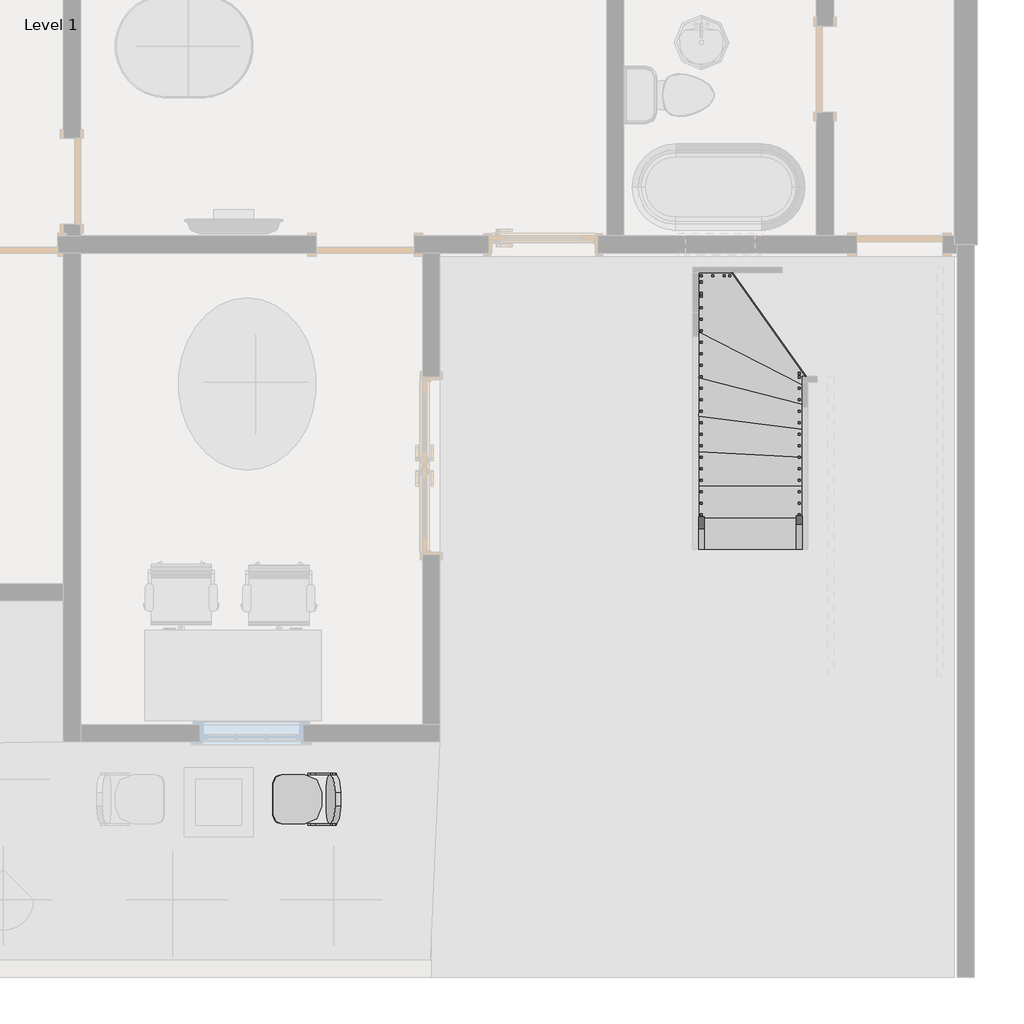
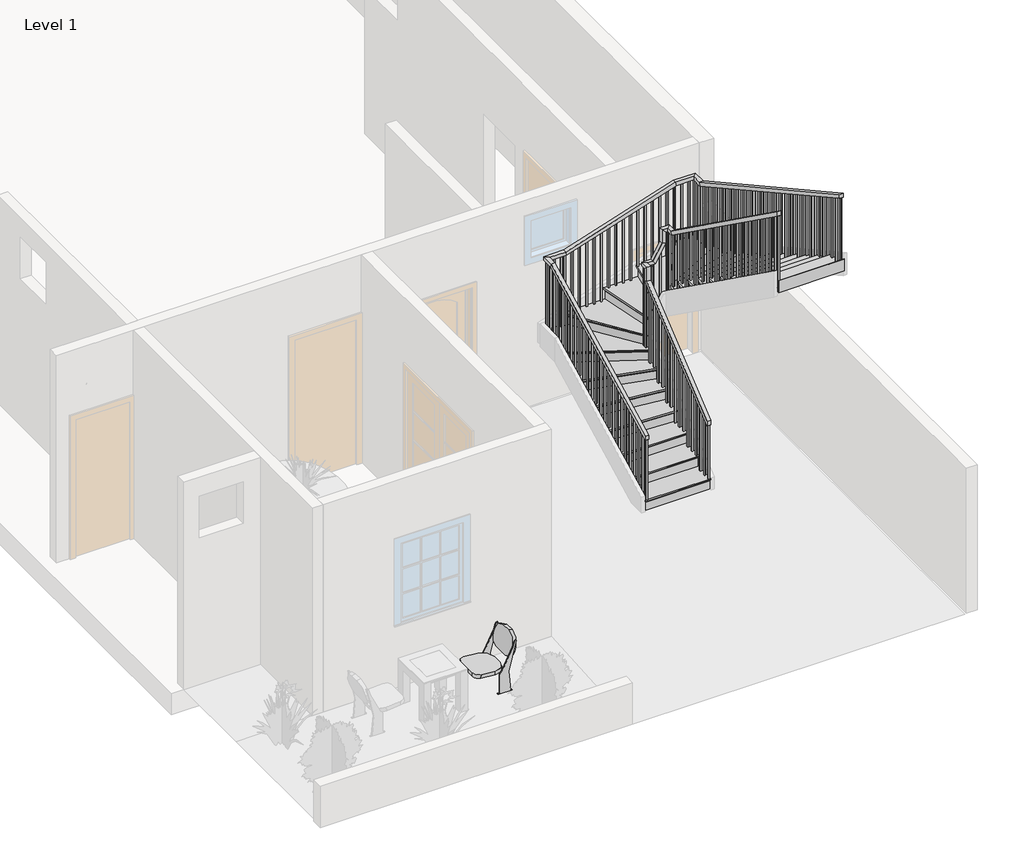
# One storey, part 2 of 3: 2 railings, 1 furniture element, 1 stair flight.
"""IFC4 building model written with IfcOpenShell, lengths in millimetres."""

from ifc_helpers import new_model, si_unit, frame, origin, place, context, project, spatial, polyline, outline, extrude, faceted_brep, transform, mapped, element, save
from components import furniture_3d1d9cbc, stair_flight_43e61283

model = new_model("IFC4")

# Units and contexts
model_context = context("Model", 3, world=origin())
ifc_project = project(units=[si_unit("LENGTHUNIT", "METRE", prefix="MILLI")], contexts=[model_context])

# Site, building, storey
site = spatial("IfcSite", under=ifc_project)
building = spatial("IfcBuilding", under=site)
storey = spatial("IfcBuildingStorey", under=building, Name="Level 1", Elevation=0.0)

# Furniture
placement = place(None, origin())
furniture_shape = furniture_3d1d9cbc(model_context)
element("IfcFurniture", 1, ObjectType="Seating-Auditorium : 18\" x 24\" x 30\"", at=placement, inside=storey, context=model_context, shape_type="MappedRepresentation", body=[
    mapped(furniture_shape, transform((-11062.1267733, -4008.1174688, 0.0), x_axis=(0.0, 1.0, 0.0), y_axis=(-1.0, 0.0, 0.0), z_axis=(0.0, 0.0, 1.0))),
])

# Railings
element("IfcRailing", 2, ObjectType="Handrail - Rectangular", at=placement, inside=storey, context=model_context, shape_type="SolidModel", body=[
    faceted_brep([(-6934.0021832, -1637.5895999, 1025.2529681), (-6934.0021832, -1637.5895999, 959.7067088), (-6883.2021832, -1637.5895999, 959.7067088), (-6883.2021832, -1637.5895999, 1025.2529681), (-6934.0021832, -186.057908, 2208.7848338), (-6934.0021832, -135.257908, 2184.659247), (-6883.2021832, -135.257908, 2184.659247), (-6883.2021832, -186.057908, 2208.7848338), (-6934.0021832, -186.057908, 2414.6281882), (-6934.0021832, -135.257908, 2363.8281882), (-6883.2021832, -135.257908, 2363.8281882), (-6883.2021832, -186.057908, 2414.6281882), (-6934.0021832, -59.057908, 2414.6281882), (-6934.0021832, -59.057908, 2363.8281882), (-6883.2021832, -109.857908, 2363.8281882), (-6883.2021832, -109.857908, 2414.6281882), (-6807.0021832, -59.057908, 2414.6281882), (-6777.8808493, -59.057908, 2363.8281882), (-6777.8808493, -109.857908, 2363.8281882), (-6807.0021832, -109.857908, 2414.6281882), (-6680.0021832, -59.057908, 2631.5051451), (-6629.2021832, -59.057908, 2617.7256424), (-6629.2021832, -109.857908, 2617.7256424), (-6680.0021832, -109.857908, 2631.5051451), (-6680.0021832, -59.057908, 2830.0317636), (-6629.2021832, -59.057908, 2779.2317636), (-6629.2021832, -109.857908, 2779.2317636), (-6680.0021832, -109.857908, 2830.0317636), (-6553.0021832, -59.057908, 2830.0317636), (-6553.0021832, -59.057908, 2779.2317636), (-6603.8021832, -109.857908, 2779.2317636), (-6603.8021832, -109.857908, 2830.0317636), (-6553.0021832, -186.057908, 2830.0317636), (-6553.0021832, -202.3767503, 2779.2317636), (-6603.8021832, -202.3767503, 2779.2317636), (-6603.8021832, -186.057908, 2830.0317636), (-6553.0021832, -2755.1895999, 4670.5627033), (-6603.8021832, -2755.1895999, 4670.5627033), (-6603.8021832, -2755.1895999, 4608.071853), (-6553.0021832, -2755.1895999, 4608.071853)], [[[0, 1, 2, 3]], [[1, 0, 4, 5]], [[2, 1, 5, 6]], [[3, 2, 6, 7]], [[0, 3, 7, 4]], [[5, 4, 8, 9]], [[6, 5, 9, 10]], [[7, 6, 10, 11]], [[4, 7, 11, 8]], [[9, 8, 12, 13]], [[10, 9, 13, 14]], [[11, 10, 14, 15]], [[8, 11, 15, 12]], [[13, 12, 16, 17]], [[14, 13, 17, 18]], [[15, 14, 18, 19]], [[12, 15, 19, 16]], [[17, 16, 20, 21]], [[18, 17, 21, 22]], [[19, 18, 22, 23]], [[16, 19, 23, 20]], [[21, 20, 24, 25]], [[22, 21, 25, 26]], [[23, 22, 26, 27]], [[20, 23, 27, 24]], [[25, 24, 28, 29]], [[26, 25, 29, 30]], [[27, 26, 30, 31]], [[24, 27, 31, 28]], [[29, 28, 32, 33]], [[30, 29, 33, 34]], [[31, 30, 34, 35]], [[28, 31, 35, 32]], [[36, 37, 38, 39]], [[33, 32, 36, 39]], [[34, 33, 39, 38]], [[35, 34, 38, 37]], [[32, 35, 37, 36]]]),
    extrude(outline(polyline([(-2667.3171173, 4545.1198356), (-2648.2671173, 4531.4723785), (-2648.2671173, 3556.0), (-2667.3171173, 3556.0), (-2667.3171173, 4545.1198356)])), frame((-6587.9271832, 0.0, 0.0), z_axis=(1.0, 0.0, 0.0), x_axis=(0.0, 1.0, 0.0)), (0.0, 0.0, 1.0), 19.05),
    extrude(outline(polyline([(-2565.7171173, 4472.333398), (-2546.6671173, 4458.685941), (-2546.6671173, 3556.0), (-2565.7171173, 3556.0), (-2565.7171173, 4472.333398)])), frame((-6587.9271832, 0.0, 0.0), z_axis=(1.0, 0.0, 0.0), x_axis=(0.0, 1.0, 0.0)), (0.0, 0.0, 1.0), 19.05),
    extrude(outline(polyline([(-2464.1171173, 4399.5469605), (-2445.0671173, 4385.8995034), (-2445.0671173, 3386.6666667), (-2464.1171173, 3386.6666667), (-2464.1171173, 4399.5469605)])), frame((-6587.9271832, 0.0, 0.0), z_axis=(1.0, 0.0, 0.0), x_axis=(0.0, 1.0, 0.0)), (0.0, 0.0, 1.0), 19.05),
    extrude(outline(polyline([(-2362.5171173, 4326.7605229), (-2343.4671173, 4313.1130658), (-2343.4671173, 3386.6666667), (-2362.5171173, 3386.6666667), (-2362.5171173, 4326.7605229)])), frame((-6587.9271832, 0.0, 0.0), z_axis=(1.0, 0.0, 0.0), x_axis=(0.0, 1.0, 0.0)), (0.0, 0.0, 1.0), 19.05),
    extrude(outline(polyline([(-2260.9171173, 4253.9740853), (-2241.8671173, 4240.3266283), (-2241.8671173, 3386.6666667), (-2260.9171173, 3386.6666667), (-2260.9171173, 4253.9740853)])), frame((-6587.9271832, 0.0, 0.0), z_axis=(1.0, 0.0, 0.0), x_axis=(0.0, 1.0, 0.0)), (0.0, 0.0, 1.0), 19.05),
    extrude(outline(polyline([(-2159.3171173, 4181.1876478), (-2140.2671173, 4167.5401907), (-2140.2671173, 3217.3333333), (-2159.3171173, 3217.3333333), (-2159.3171173, 4181.1876478)])), frame((-6587.9271832, 0.0, 0.0), z_axis=(1.0, 0.0, 0.0), x_axis=(0.0, 1.0, 0.0)), (0.0, 0.0, 1.0), 19.05),
    extrude(outline(polyline([(-2057.7171173, 4108.4012102), (-2038.6671173, 4094.7537532), (-2038.6671173, 3217.3333333), (-2057.7171173, 3217.3333333), (-2057.7171173, 4108.4012102)])), frame((-6587.9271832, 0.0, 0.0), z_axis=(1.0, 0.0, 0.0), x_axis=(0.0, 1.0, 0.0)), (0.0, 0.0, 1.0), 19.05),
    extrude(outline(polyline([(-1956.1171173, 4035.6147727), (-1937.0671173, 4021.9673156), (-1937.0671173, 3217.3333333), (-1956.1171173, 3217.3333333), (-1956.1171173, 4035.6147727)])), frame((-6587.9271832, 0.0, 0.0), z_axis=(1.0, 0.0, 0.0), x_axis=(0.0, 1.0, 0.0)), (0.0, 0.0, 1.0), 19.05),
    extrude(outline(polyline([(-1854.5171173, 3962.8283351), (-1835.4671173, 3949.1808781), (-1835.4671173, 3048.0), (-1854.5171173, 3048.0), (-1854.5171173, 3962.8283351)])), frame((-6587.9271832, 0.0, 0.0), z_axis=(1.0, 0.0, 0.0), x_axis=(0.0, 1.0, 0.0)), (0.0, 0.0, 1.0), 19.05),
    extrude(outline(polyline([(-1752.9171173, 3890.0418975), (-1733.8671173, 3876.3944405), (-1733.8671173, 3048.0), (-1752.9171173, 3048.0), (-1752.9171173, 3890.0418975)])), frame((-6587.9271832, 0.0, 0.0), z_axis=(1.0, 0.0, 0.0), x_axis=(0.0, 1.0, 0.0)), (0.0, 0.0, 1.0), 19.05),
    extrude(outline(polyline([(-1651.3171173, 3817.25546), (-1632.2671173, 3803.6080029), (-1632.2671173, 2878.6666667), (-1651.3171173, 2878.6666667), (-1651.3171173, 3817.25546)])), frame((-6587.9271832, 0.0, 0.0), z_axis=(1.0, 0.0, 0.0), x_axis=(0.0, 1.0, 0.0)), (0.0, 0.0, 1.0), 19.05),
    extrude(outline(polyline([(-1549.7171173, 3744.4690224), (-1530.6671173, 3730.8215654), (-1530.6671173, 2878.6666667), (-1549.7171173, 2878.6666667), (-1549.7171173, 3744.4690224)])), frame((-6587.9271832, 0.0, 0.0), z_axis=(1.0, 0.0, 0.0), x_axis=(0.0, 1.0, 0.0)), (0.0, 0.0, 1.0), 19.05),
    extrude(outline(polyline([(-1448.1171173, 3671.6825849), (-1429.0671173, 3658.0351278), (-1429.0671173, 2878.6666667), (-1448.1171173, 2878.6666667), (-1448.1171173, 3671.6825849)])), frame((-6587.9271832, 0.0, 0.0), z_axis=(1.0, 0.0, 0.0), x_axis=(0.0, 1.0, 0.0)), (0.0, 0.0, 1.0), 19.05),
    extrude(outline(polyline([(-1346.5171173, 3598.8961473), (-1327.4671173, 3585.2486903), (-1327.4671173, 2709.3333333), (-1346.5171173, 2709.3333333), (-1346.5171173, 3598.8961473)])), frame((-6587.9271832, 0.0, 0.0), z_axis=(1.0, 0.0, 0.0), x_axis=(0.0, 1.0, 0.0)), (0.0, 0.0, 1.0), 19.05),
    extrude(outline(polyline([(-1244.9171173, 3526.1097097), (-1225.8671173, 3512.4622527), (-1225.8671173, 2709.3333333), (-1244.9171173, 2709.3333333), (-1244.9171173, 3526.1097097)])), frame((-6587.9271832, 0.0, 0.0), z_axis=(1.0, 0.0, 0.0), x_axis=(0.0, 1.0, 0.0)), (0.0, 0.0, 1.0), 19.05),
    extrude(outline(polyline([(-1143.3171173, 3453.3232722), (-1124.2671173, 3439.6758151), (-1124.2671173, 2709.3333333), (-1143.3171173, 2709.3333333), (-1143.3171173, 3453.3232722)])), frame((-6587.9271832, 0.0, 0.0), z_axis=(1.0, 0.0, 0.0), x_axis=(0.0, 1.0, 0.0)), (0.0, 0.0, 1.0), 19.05),
    extrude(outline(polyline([(-1041.7171173, 3380.5368346), (-1022.6671173, 3366.8893776), (-1022.6671173, 2540.0), (-1041.7171173, 2540.0), (-1041.7171173, 3380.5368346)])), frame((-6587.9271832, 0.0, 0.0), z_axis=(1.0, 0.0, 0.0), x_axis=(0.0, 1.0, 0.0)), (0.0, 0.0, 1.0), 19.05),
    extrude(outline(polyline([(-940.1171173, 3307.7503971), (-921.0671173, 3294.10294), (-921.0671173, 2540.0), (-940.1171173, 2540.0), (-940.1171173, 3307.7503971)])), frame((-6587.9271832, 0.0, 0.0), z_axis=(1.0, 0.0, 0.0), x_axis=(0.0, 1.0, 0.0)), (0.0, 0.0, 1.0), 19.05),
    extrude(outline(polyline([(-838.5171173, 3234.9639595), (-819.4671173, 3221.3165025), (-819.4671173, 2370.6666667), (-838.5171173, 2370.6666667), (-838.5171173, 3234.9639595)])), frame((-6587.9271832, 0.0, 0.0), z_axis=(1.0, 0.0, 0.0), x_axis=(0.0, 1.0, 0.0)), (0.0, 0.0, 1.0), 19.05),
    extrude(outline(polyline([(-736.9171173, 3162.1775219), (-717.8671173, 3148.5300649), (-717.8671173, 2370.6666667), (-736.9171173, 2370.6666667), (-736.9171173, 3162.1775219)])), frame((-6587.9271832, 0.0, 0.0), z_axis=(1.0, 0.0, 0.0), x_axis=(0.0, 1.0, 0.0)), (0.0, 0.0, 1.0), 19.05),
    extrude(outline(polyline([(-635.3171173, 3089.3910844), (-616.2671173, 3075.7436273), (-616.2671173, 2370.6666667), (-635.3171173, 2370.6666667), (-635.3171173, 3089.3910844)])), frame((-6587.9271832, 0.0, 0.0), z_axis=(1.0, 0.0, 0.0), x_axis=(0.0, 1.0, 0.0)), (0.0, 0.0, 1.0), 19.05),
    extrude(outline(polyline([(-533.7171173, 3016.6046468), (-514.6671173, 3002.9571898), (-514.6671173, 2201.3333333), (-533.7171173, 2201.3333333), (-533.7171173, 3016.6046468)])), frame((-6587.9271832, 0.0, 0.0), z_axis=(1.0, 0.0, 0.0), x_axis=(0.0, 1.0, 0.0)), (0.0, 0.0, 1.0), 19.05),
    extrude(outline(polyline([(-432.1171173, 2943.8182093), (-413.0671173, 2930.1707522), (-413.0671173, 2201.3333333), (-432.1171173, 2201.3333333), (-432.1171173, 2943.8182093)])), frame((-6587.9271832, 0.0, 0.0), z_axis=(1.0, 0.0, 0.0), x_axis=(0.0, 1.0, 0.0)), (0.0, 0.0, 1.0), 19.05),
    extrude(outline(polyline([(-330.5171173, 2871.0317717), (-311.4671173, 2857.3843147), (-311.4671173, 2032.0), (-330.5171173, 2032.0), (-330.5171173, 2871.0317717)])), frame((-6587.9271832, 0.0, 0.0), z_axis=(1.0, 0.0, 0.0), x_axis=(0.0, 1.0, 0.0)), (0.0, 0.0, 1.0), 19.05),
    extrude(outline(polyline([(-228.9171173, 2798.2453341), (-209.8671173, 2784.5978771), (-209.8671173, 2032.0), (-228.9171173, 2032.0), (-228.9171173, 2798.2453341)])), frame((-6587.9271832, 0.0, 0.0), z_axis=(1.0, 0.0, 0.0), x_axis=(0.0, 1.0, 0.0)), (0.0, 0.0, 1.0), 19.05),
    extrude(outline(polyline([(2529.115018, -6681.0912794), (2496.5834745, -6700.1412794), (1524.0, -6700.1412794), (1524.0, -6681.0912794), (2529.115018, -6681.0912794)])), frame((0.0, -93.982908, 0.0), z_axis=(0.0, 1.0, 0.0), x_axis=(0.0, 0.0, 1.0)), (0.0, 0.0, 1.0), 19.05),
    extrude(outline(polyline([(2355.6134525, -6782.6912794), (2323.0819089, -6801.7412794), (1524.0, -6801.7412794), (1524.0, -6782.6912794), (2355.6134525, -6782.6912794)])), frame((0.0, -93.982908, 0.0), z_axis=(0.0, 1.0, 0.0), x_axis=(0.0, 0.0, 1.0)), (0.0, 0.0, 1.0), 19.05),
    extrude(outline(polyline([(-224.7145999, 2111.7191617), (-205.6645999, 2127.2519138), (-205.6645999, 1016.0), (-224.7145999, 1016.0), (-224.7145999, 2111.7191617)])), frame((-6918.1271832, 0.0, 0.0), z_axis=(1.0, 0.0, 0.0), x_axis=(0.0, 1.0, 0.0)), (0.0, 0.0, 1.0), 19.05),
    extrude(outline(polyline([(-326.3145999, 2028.8778167), (-307.2645999, 2044.4105689), (-307.2645999, 1016.0), (-326.3145999, 1016.0), (-326.3145999, 2028.8778167)])), frame((-6918.1271832, 0.0, 0.0), z_axis=(1.0, 0.0, 0.0), x_axis=(0.0, 1.0, 0.0)), (0.0, 0.0, 1.0), 19.05),
    extrude(outline(polyline([(-427.9145999, 1946.0364718), (-408.8645999, 1961.569224), (-408.8645999, 846.6666667), (-427.9145999, 846.6666667), (-427.9145999, 1946.0364718)])), frame((-6918.1271832, 0.0, 0.0), z_axis=(1.0, 0.0, 0.0), x_axis=(0.0, 1.0, 0.0)), (0.0, 0.0, 1.0), 19.05),
    extrude(outline(polyline([(-529.5145999, 1863.1951269), (-510.4645999, 1878.7278791), (-510.4645999, 846.6666667), (-529.5145999, 846.6666667), (-529.5145999, 1863.1951269)])), frame((-6918.1271832, 0.0, 0.0), z_axis=(1.0, 0.0, 0.0), x_axis=(0.0, 1.0, 0.0)), (0.0, 0.0, 1.0), 19.05),
    extrude(outline(polyline([(-631.1145999, 1780.353782), (-612.0645999, 1795.8865341), (-612.0645999, 677.3333333), (-631.1145999, 677.3333333), (-631.1145999, 1780.353782)])), frame((-6918.1271832, 0.0, 0.0), z_axis=(1.0, 0.0, 0.0), x_axis=(0.0, 1.0, 0.0)), (0.0, 0.0, 1.0), 19.05),
    extrude(outline(polyline([(-732.7145999, 1697.5124371), (-713.6645999, 1713.0451892), (-713.6645999, 677.3333333), (-732.7145999, 677.3333333), (-732.7145999, 1697.5124371)])), frame((-6918.1271832, 0.0, 0.0), z_axis=(1.0, 0.0, 0.0), x_axis=(0.0, 1.0, 0.0)), (0.0, 0.0, 1.0), 19.05),
    extrude(outline(polyline([(-834.3145999, 1614.6710921), (-815.2645999, 1630.2038443), (-815.2645999, 508.0), (-834.3145999, 508.0), (-834.3145999, 1614.6710921)])), frame((-6918.1271832, 0.0, 0.0), z_axis=(1.0, 0.0, 0.0), x_axis=(0.0, 1.0, 0.0)), (0.0, 0.0, 1.0), 19.05),
    extrude(outline(polyline([(-935.9145999, 1531.8297472), (-916.8645999, 1547.3624994), (-916.8645999, 508.0), (-935.9145999, 508.0), (-935.9145999, 1531.8297472)])), frame((-6918.1271832, 0.0, 0.0), z_axis=(1.0, 0.0, 0.0), x_axis=(0.0, 1.0, 0.0)), (0.0, 0.0, 1.0), 19.05),
    extrude(outline(polyline([(-1037.5145999, 1448.9884023), (-1018.4645999, 1464.5211545), (-1018.4645999, 508.0), (-1037.5145999, 508.0), (-1037.5145999, 1448.9884023)])), frame((-6918.1271832, 0.0, 0.0), z_axis=(1.0, 0.0, 0.0), x_axis=(0.0, 1.0, 0.0)), (0.0, 0.0, 1.0), 19.05),
    extrude(outline(polyline([(-1139.1145999, 1366.1470574), (-1120.0645999, 1381.6798095), (-1120.0645999, 338.6666667), (-1139.1145999, 338.6666667), (-1139.1145999, 1366.1470574)])), frame((-6918.1271832, 0.0, 0.0), z_axis=(1.0, 0.0, 0.0), x_axis=(0.0, 1.0, 0.0)), (0.0, 0.0, 1.0), 19.05),
    extrude(outline(polyline([(-1240.7145999, 1283.3057124), (-1221.6645999, 1298.8384646), (-1221.6645999, 338.6666667), (-1240.7145999, 338.6666667), (-1240.7145999, 1283.3057124)])), frame((-6918.1271832, 0.0, 0.0), z_axis=(1.0, 0.0, 0.0), x_axis=(0.0, 1.0, 0.0)), (0.0, 0.0, 1.0), 19.05),
    extrude(outline(polyline([(-1342.3145999, 1200.4643675), (-1323.2645999, 1215.9971197), (-1323.2645999, 338.6666667), (-1342.3145999, 338.6666667), (-1342.3145999, 1200.4643675)])), frame((-6918.1271832, 0.0, 0.0), z_axis=(1.0, 0.0, 0.0), x_axis=(0.0, 1.0, 0.0)), (0.0, 0.0, 1.0), 19.05),
    extrude(outline(polyline([(-1443.9145999, 1117.6230226), (-1424.8645999, 1133.1557748), (-1424.8645999, 169.3333333), (-1443.9145999, 169.3333333), (-1443.9145999, 1117.6230226)])), frame((-6918.1271832, 0.0, 0.0), z_axis=(1.0, 0.0, 0.0), x_axis=(0.0, 1.0, 0.0)), (0.0, 0.0, 1.0), 19.05),
    extrude(outline(polyline([(-1545.5145999, 1034.7816777), (-1526.4645999, 1050.3144298), (-1526.4645999, 169.3333333), (-1545.5145999, 169.3333333), (-1545.5145999, 1034.7816777)])), frame((-6918.1271832, 0.0, 0.0), z_axis=(1.0, 0.0, 0.0), x_axis=(0.0, 1.0, 0.0)), (0.0, 0.0, 1.0), 19.05),
    extrude(outline(polyline([(-6587.9271832, -108.2671173), (-6568.8771832, -108.2671173), (-6568.8771832, -127.3171173), (-6587.9271832, -127.3171173), (-6587.9271832, -108.2671173)])), frame((0.0, 0.0, 1862.6666667), z_axis=(0.0, 0.0, 1.0), x_axis=(1.0, 0.0, 0.0)), (0.0, 0.0, 1.0), 916.5650969),
    extrude(outline(polyline([(-6587.9271832, -93.982908), (-6587.9271832, -74.932908), (-6568.8771832, -74.932908), (-6568.8771832, -93.982908), (-6587.9271832, -93.982908)])), frame((0.0, 0.0, 1862.6666667), z_axis=(0.0, 0.0, 1.0), x_axis=(1.0, 0.0, 0.0)), (0.0, 0.0, 1.0), 916.5650969),
    extrude(outline(polyline([(-6601.9113702, -93.982908), (-6601.9113702, -74.932908), (-6582.8613702, -74.932908), (-6582.8613702, -93.982908), (-6601.9113702, -93.982908)])), frame((0.0, 0.0, 1693.3333333), z_axis=(0.0, 0.0, 1.0), x_axis=(1.0, 0.0, 0.0)), (0.0, 0.0, 1.0), 1085.8984303),
    extrude(outline(polyline([(-6903.3412794, -93.982908), (-6903.3412794, -74.932908), (-6884.2912794, -74.932908), (-6884.2912794, -93.982908), (-6903.3412794, -93.982908)])), frame((0.0, 0.0, 1354.6666667), z_axis=(0.0, 0.0, 1.0), x_axis=(1.0, 0.0, 0.0)), (0.0, 0.0, 1.0), 1009.1615215),
    extrude(outline(polyline([(-6899.0771832, -93.982908), (-6918.1271832, -93.982908), (-6918.1271832, -74.932908), (-6899.0771832, -74.932908), (-6899.0771832, -93.982908)])), frame((0.0, 0.0, 1185.3333333), z_axis=(0.0, 0.0, 1.0), x_axis=(1.0, 0.0, 0.0)), (0.0, 0.0, 1.0), 1178.4948549),
    extrude(outline(polyline([(-6899.0771832, -124.9502644), (-6918.1271832, -124.9502644), (-6918.1271832, -105.9002644), (-6899.0771832, -105.9002644), (-6899.0771832, -124.9502644)])), frame((0.0, 0.0, 1185.3333333), z_axis=(0.0, 0.0, 1.0), x_axis=(1.0, 0.0, 0.0)), (0.0, 0.0, 1.0), 1178.4948549),
    extrude(outline(polyline([(-2755.1895999, 4608.071853), (-2736.1395999, 4594.4243959), (-2736.1395999, 3556.0), (-2755.1895999, 3556.0), (-2755.1895999, 4608.071853)])), frame((-6587.9271832, 0.0, 0.0), z_axis=(1.0, 0.0, 0.0), x_axis=(0.0, 1.0, 0.0)), (0.0, 0.0, 1.0), 19.05),
    extrude(outline(polyline([(-1637.5895999, 959.7067088), (-1618.5395999, 975.239461), (-1618.5395999, 169.3333333), (-1637.5895999, 169.3333333), (-1637.5895999, 959.7067088)])), frame((-6918.1271832, 0.0, 0.0), z_axis=(1.0, 0.0, 0.0), x_axis=(0.0, 1.0, 0.0)), (0.0, 0.0, 1.0), 19.05),
])
element("IfcRailing", 3, ObjectType="Handrail - Rectangular", at=placement, inside=storey, context=model_context, shape_type="SolidModel", body=[
    faceted_brep([(-7797.6021832, -1637.5895999, 1109.0771751), (-7797.6021832, -1637.5895999, 1051.9280057), (-7746.8021832, -1637.5895999, 1051.9280057), (-7746.8021832, -1637.5895999, 1109.0771751), (-7797.6021832, 622.3922566, 2273.7644996), (-7797.6021832, 634.7123079, 2222.9644996), (-7746.8021832, 634.7123079, 2222.9644996), (-7746.8021832, 622.3922566, 2273.7644996), (-7797.6021832, 804.542092, 2273.7644996), (-7797.6021832, 804.542092, 2222.9644996), (-7746.8021832, 753.742092, 2222.9644996), (-7746.8021832, 753.742092, 2273.7644996), (-7520.4482306, 804.542092, 2273.7644996), (-7512.4976544, 804.542092, 2222.9644996), (-7512.4976544, 753.742092, 2222.9644996), (-7520.4482306, 753.742092, 2273.7644996), (-5994.850361, 804.542092, 2763.2899386), (-5986.8997849, 804.542092, 2712.4899386), (-5986.8997849, 753.742092, 2712.4899386), (-5994.850361, 753.742092, 2763.2899386), (-5689.4021832, 804.542092, 2763.2899386), (-5689.4021832, 804.542092, 2712.4899386), (-5740.2021832, 753.742092, 2712.4899386), (-5740.2021832, 753.742092, 2763.2899386), (-5689.4021832, 616.3741381, 2763.2899386), (-5689.4021832, 603.282684, 2712.4899386), (-5740.2021832, 603.282684, 2712.4899386), (-5740.2021832, 616.3741381, 2763.2899386), (-5689.4021832, -2755.1895999, 4624.6500953), (-5740.2021832, -2755.1895999, 4624.6500953), (-5740.2021832, -2755.1895999, 4566.6226148), (-5689.4021832, -2755.1895999, 4566.6226148)], [[[0, 1, 2, 3]], [[1, 0, 4, 5]], [[2, 1, 5, 6]], [[3, 2, 6, 7]], [[0, 3, 7, 4]], [[5, 4, 8, 9]], [[6, 5, 9, 10]], [[7, 6, 10, 11]], [[4, 7, 11, 8]], [[9, 8, 12, 13]], [[10, 9, 13, 14]], [[11, 10, 14, 15]], [[8, 11, 15, 12]], [[13, 12, 16, 17]], [[14, 13, 17, 18]], [[15, 14, 18, 19]], [[12, 15, 19, 16]], [[17, 16, 20, 21]], [[18, 17, 21, 22]], [[19, 18, 22, 23]], [[16, 19, 23, 20]], [[21, 20, 24, 25]], [[22, 21, 25, 26]], [[23, 22, 26, 27]], [[20, 23, 27, 24]], [[28, 29, 30, 31]], [[25, 24, 28, 31]], [[26, 25, 31, 30]], [[27, 26, 30, 29]], [[24, 27, 29, 28]]]),
    extrude(outline(polyline([(-2726.9008619, 4551.0050753), (-2726.9008619, 3556.0), (-2745.9508619, 3556.0), (-2745.9508619, 4561.5221272), (-2726.9008619, 4551.0050753)])), frame((-5724.3271832, 0.0, 0.0), z_axis=(1.0, 0.0, 0.0), x_axis=(0.0, 1.0, 0.0)), (0.0, 0.0, 1.0), 19.05),
    extrude(outline(polyline([(-2625.3008619, 4494.9141316), (-2625.3008619, 3556.0), (-2644.3508619, 3556.0), (-2644.3508619, 4505.4311835), (-2625.3008619, 4494.9141316)])), frame((-5724.3271832, 0.0, 0.0), z_axis=(1.0, 0.0, 0.0), x_axis=(0.0, 1.0, 0.0)), (0.0, 0.0, 1.0), 19.05),
    extrude(outline(polyline([(-2523.7008619, 4438.8231878), (-2523.7008619, 3556.0), (-2542.7508619, 3556.0), (-2542.7508619, 4449.3402398), (-2523.7008619, 4438.8231878)])), frame((-5724.3271832, 0.0, 0.0), z_axis=(1.0, 0.0, 0.0), x_axis=(0.0, 1.0, 0.0)), (0.0, 0.0, 1.0), 19.05),
    extrude(outline(polyline([(-2422.1008619, 4382.7322441), (-2422.1008619, 3386.6666667), (-2441.1508619, 3386.6666667), (-2441.1508619, 4393.249296), (-2422.1008619, 4382.7322441)])), frame((-5724.3271832, 0.0, 0.0), z_axis=(1.0, 0.0, 0.0), x_axis=(0.0, 1.0, 0.0)), (0.0, 0.0, 1.0), 19.05),
    extrude(outline(polyline([(-2320.5008619, 4326.6413004), (-2320.5008619, 3386.6666667), (-2339.5508619, 3386.6666667), (-2339.5508619, 4337.1583523), (-2320.5008619, 4326.6413004)])), frame((-5724.3271832, 0.0, 0.0), z_axis=(1.0, 0.0, 0.0), x_axis=(0.0, 1.0, 0.0)), (0.0, 0.0, 1.0), 19.05),
    extrude(outline(polyline([(-2218.9008619, 4270.5503566), (-2218.9008619, 3386.6666667), (-2237.9508619, 3386.6666667), (-2237.9508619, 4281.0674086), (-2218.9008619, 4270.5503566)])), frame((-5724.3271832, 0.0, 0.0), z_axis=(1.0, 0.0, 0.0), x_axis=(0.0, 1.0, 0.0)), (0.0, 0.0, 1.0), 19.05),
    extrude(outline(polyline([(-2117.3008619, 4214.4594129), (-2117.3008619, 3217.3333333), (-2136.3508619, 3217.3333333), (-2136.3508619, 4224.9764648), (-2117.3008619, 4214.4594129)])), frame((-5724.3271832, 0.0, 0.0), z_axis=(1.0, 0.0, 0.0), x_axis=(0.0, 1.0, 0.0)), (0.0, 0.0, 1.0), 19.05),
    extrude(outline(polyline([(-2015.7008619, 4158.3684692), (-2015.7008619, 3217.3333333), (-2034.7508619, 3217.3333333), (-2034.7508619, 4168.8855211), (-2015.7008619, 4158.3684692)])), frame((-5724.3271832, 0.0, 0.0), z_axis=(1.0, 0.0, 0.0), x_axis=(0.0, 1.0, 0.0)), (0.0, 0.0, 1.0), 19.05),
    extrude(outline(polyline([(-1914.1008619, 4102.2775254), (-1914.1008619, 3217.3333333), (-1933.1508619, 3217.3333333), (-1933.1508619, 4112.7945774), (-1914.1008619, 4102.2775254)])), frame((-5724.3271832, 0.0, 0.0), z_axis=(1.0, 0.0, 0.0), x_axis=(0.0, 1.0, 0.0)), (0.0, 0.0, 1.0), 19.05),
    extrude(outline(polyline([(-1812.5008619, 4046.1865817), (-1812.5008619, 3048.0), (-1831.5508619, 3048.0), (-1831.5508619, 4056.7036337), (-1812.5008619, 4046.1865817)])), frame((-5724.3271832, 0.0, 0.0), z_axis=(1.0, 0.0, 0.0), x_axis=(0.0, 1.0, 0.0)), (0.0, 0.0, 1.0), 19.05),
    extrude(outline(polyline([(-1710.9008619, 3990.095638), (-1710.9008619, 3048.0), (-1729.9508619, 3048.0), (-1729.9508619, 4000.6126899), (-1710.9008619, 3990.095638)])), frame((-5724.3271832, 0.0, 0.0), z_axis=(1.0, 0.0, 0.0), x_axis=(0.0, 1.0, 0.0)), (0.0, 0.0, 1.0), 19.05),
    extrude(outline(polyline([(-1609.3008619, 3934.0046942), (-1609.3008619, 2878.6666667), (-1628.3508619, 2878.6666667), (-1628.3508619, 3944.5217462), (-1609.3008619, 3934.0046942)])), frame((-5724.3271832, 0.0, 0.0), z_axis=(1.0, 0.0, 0.0), x_axis=(0.0, 1.0, 0.0)), (0.0, 0.0, 1.0), 19.05),
    extrude(outline(polyline([(-1507.7008619, 3877.9137505), (-1507.7008619, 2878.6666667), (-1526.7508619, 2878.6666667), (-1526.7508619, 3888.4308025), (-1507.7008619, 3877.9137505)])), frame((-5724.3271832, 0.0, 0.0), z_axis=(1.0, 0.0, 0.0), x_axis=(0.0, 1.0, 0.0)), (0.0, 0.0, 1.0), 19.05),
    extrude(outline(polyline([(-1406.1008619, 3821.8228068), (-1406.1008619, 2878.6666667), (-1425.1508619, 2878.6666667), (-1425.1508619, 3832.3398587), (-1406.1008619, 3821.8228068)])), frame((-5724.3271832, 0.0, 0.0), z_axis=(1.0, 0.0, 0.0), x_axis=(0.0, 1.0, 0.0)), (0.0, 0.0, 1.0), 19.05),
    extrude(outline(polyline([(-1304.5008619, 3765.731863), (-1304.5008619, 2709.3333333), (-1323.5508619, 2709.3333333), (-1323.5508619, 3776.248915), (-1304.5008619, 3765.731863)])), frame((-5724.3271832, 0.0, 0.0), z_axis=(1.0, 0.0, 0.0), x_axis=(0.0, 1.0, 0.0)), (0.0, 0.0, 1.0), 19.05),
    extrude(outline(polyline([(-1202.9008619, 3709.6409193), (-1202.9008619, 2709.3333333), (-1221.9508619, 2709.3333333), (-1221.9508619, 3720.1579713), (-1202.9008619, 3709.6409193)])), frame((-5724.3271832, 0.0, 0.0), z_axis=(1.0, 0.0, 0.0), x_axis=(0.0, 1.0, 0.0)), (0.0, 0.0, 1.0), 19.05),
    extrude(outline(polyline([(-1101.3008619, 3653.5499756), (-1101.3008619, 2709.3333333), (-1120.3508619, 2709.3333333), (-1120.3508619, 3664.0670275), (-1101.3008619, 3653.5499756)])), frame((-5724.3271832, 0.0, 0.0), z_axis=(1.0, 0.0, 0.0), x_axis=(0.0, 1.0, 0.0)), (0.0, 0.0, 1.0), 19.05),
    extrude(outline(polyline([(-999.7008619, 3597.4590319), (-999.7008619, 2540.0), (-1018.7508619, 2540.0), (-1018.7508619, 3607.9760838), (-999.7008619, 3597.4590319)])), frame((-5724.3271832, 0.0, 0.0), z_axis=(1.0, 0.0, 0.0), x_axis=(0.0, 1.0, 0.0)), (0.0, 0.0, 1.0), 19.05),
    extrude(outline(polyline([(-898.1008619, 3541.3680881), (-898.1008619, 2540.0), (-917.1508619, 2540.0), (-917.1508619, 3551.8851401), (-898.1008619, 3541.3680881)])), frame((-5724.3271832, 0.0, 0.0), z_axis=(1.0, 0.0, 0.0), x_axis=(0.0, 1.0, 0.0)), (0.0, 0.0, 1.0), 19.05),
    extrude(outline(polyline([(-796.5008619, 3485.2771444), (-796.5008619, 2540.0), (-815.5508619, 2540.0), (-815.5508619, 3495.7941963), (-796.5008619, 3485.2771444)])), frame((-5724.3271832, 0.0, 0.0), z_axis=(1.0, 0.0, 0.0), x_axis=(0.0, 1.0, 0.0)), (0.0, 0.0, 1.0), 19.05),
    extrude(outline(polyline([(-694.9008619, 3429.1862007), (-694.9008619, 2370.6666667), (-713.9508619, 2370.6666667), (-713.9508619, 3439.7032526), (-694.9008619, 3429.1862007)])), frame((-5724.3271832, 0.0, 0.0), z_axis=(1.0, 0.0, 0.0), x_axis=(0.0, 1.0, 0.0)), (0.0, 0.0, 1.0), 19.05),
    extrude(outline(polyline([(-593.3008619, 3373.0952569), (-593.3008619, 2370.6666667), (-612.3508619, 2370.6666667), (-612.3508619, 3383.6123089), (-593.3008619, 3373.0952569)])), frame((-5724.3271832, 0.0, 0.0), z_axis=(1.0, 0.0, 0.0), x_axis=(0.0, 1.0, 0.0)), (0.0, 0.0, 1.0), 19.05),
    extrude(outline(polyline([(-491.7008619, 3317.0043132), (-491.7008619, 2370.6666667), (-510.7508619, 2370.6666667), (-510.7508619, 3327.5213651), (-491.7008619, 3317.0043132)])), frame((-5724.3271832, 0.0, 0.0), z_axis=(1.0, 0.0, 0.0), x_axis=(0.0, 1.0, 0.0)), (0.0, 0.0, 1.0), 19.05),
    extrude(outline(polyline([(-390.1008619, 3260.9133695), (-390.1008619, 2201.3333333), (-409.1508619, 2201.3333333), (-409.1508619, 3271.4304214), (-390.1008619, 3260.9133695)])), frame((-5724.3271832, 0.0, 0.0), z_axis=(1.0, 0.0, 0.0), x_axis=(0.0, 1.0, 0.0)), (0.0, 0.0, 1.0), 19.05),
    extrude(outline(polyline([(-288.5008619, 3204.8224257), (-288.5008619, 2201.3333333), (-307.5508619, 2201.3333333), (-307.5508619, 3215.3394777), (-288.5008619, 3204.8224257)])), frame((-5724.3271832, 0.0, 0.0), z_axis=(1.0, 0.0, 0.0), x_axis=(0.0, 1.0, 0.0)), (0.0, 0.0, 1.0), 19.05),
    extrude(outline(polyline([(-186.9008619, 3148.731482), (-186.9008619, 2201.3333333), (-205.9508619, 2201.3333333), (-205.9508619, 3159.248534), (-186.9008619, 3148.731482)])), frame((-5724.3271832, 0.0, 0.0), z_axis=(1.0, 0.0, 0.0), x_axis=(0.0, 1.0, 0.0)), (0.0, 0.0, 1.0), 19.05),
    extrude(outline(polyline([(-85.3008619, 3092.6405383), (-85.3008619, 2032.0), (-104.3508619, 2032.0), (-104.3508619, 3103.1575902), (-85.3008619, 3092.6405383)])), frame((-5724.3271832, 0.0, 0.0), z_axis=(1.0, 0.0, 0.0), x_axis=(0.0, 1.0, 0.0)), (0.0, 0.0, 1.0), 19.05),
    extrude(outline(polyline([(16.2991381, 3036.5495945), (16.2991381, 2032.0), (-2.7508619, 2032.0), (-2.7508619, 3047.0666465), (16.2991381, 3036.5495945)])), frame((-5724.3271832, 0.0, 0.0), z_axis=(1.0, 0.0, 0.0), x_axis=(0.0, 1.0, 0.0)), (0.0, 0.0, 1.0), 19.05),
    extrude(outline(polyline([(117.8991381, 2980.4586508), (117.8991381, 2032.0), (98.8491381, 2032.0), (98.8491381, 2990.9757028), (117.8991381, 2980.4586508)])), frame((-5724.3271832, 0.0, 0.0), z_axis=(1.0, 0.0, 0.0), x_axis=(0.0, 1.0, 0.0)), (0.0, 0.0, 1.0), 19.05),
    extrude(outline(polyline([(219.4991381, 2924.3677071), (219.4991381, 2032.0), (200.4491381, 2032.0), (200.4491381, 2934.884759), (219.4991381, 2924.3677071)])), frame((-5724.3271832, 0.0, 0.0), z_axis=(1.0, 0.0, 0.0), x_axis=(0.0, 1.0, 0.0)), (0.0, 0.0, 1.0), 19.05),
    extrude(outline(polyline([(321.0991381, 2868.2767633), (321.0991381, 1862.6666667), (302.0491381, 1862.6666667), (302.0491381, 2878.7938153), (321.0991381, 2868.2767633)])), frame((-5724.3271832, 0.0, 0.0), z_axis=(1.0, 0.0, 0.0), x_axis=(0.0, 1.0, 0.0)), (0.0, 0.0, 1.0), 19.05),
    extrude(outline(polyline([(422.6991381, 2812.1858196), (422.6991381, 1862.6666667), (403.6491381, 1862.6666667), (403.6491381, 2822.7028716), (422.6991381, 2812.1858196)])), frame((-5724.3271832, 0.0, 0.0), z_axis=(1.0, 0.0, 0.0), x_axis=(0.0, 1.0, 0.0)), (0.0, 0.0, 1.0), 19.05),
    extrude(outline(polyline([(524.2991381, 2756.0948759), (524.2991381, 1862.6666667), (505.2491381, 1862.6666667), (505.2491381, 2766.6119278), (524.2991381, 2756.0948759)])), frame((-5724.3271832, 0.0, 0.0), z_axis=(1.0, 0.0, 0.0), x_axis=(0.0, 1.0, 0.0)), (0.0, 0.0, 1.0), 19.05),
    extrude(outline(polyline([(-5705.2771832, 687.067092), (-5705.2771832, 668.017092), (-5724.3271832, 668.017092), (-5724.3271832, 687.067092), (-5705.2771832, 687.067092)])), frame((0.0, 0.0, 1862.6666667), z_axis=(0.0, 0.0, 1.0), x_axis=(1.0, 0.0, 0.0)), (0.0, 0.0, 1.0), 849.8232719),
    extrude(outline(polyline([(-5801.175361, 788.667092), (-5782.125361, 788.667092), (-5782.125361, 769.617092), (-5801.175361, 769.617092), (-5801.175361, 788.667092)])), frame((0.0, 0.0, 1862.6666667), z_axis=(0.0, 0.0, 1.0), x_axis=(1.0, 0.0, 0.0)), (0.0, 0.0, 1.0), 849.8232719),
    extrude(outline(polyline([(-5902.775361, 788.667092), (-5883.725361, 788.667092), (-5883.725361, 769.617092), (-5902.775361, 769.617092), (-5902.775361, 788.667092)])), frame((0.0, 0.0, 1862.6666667), z_axis=(0.0, 0.0, 1.0), x_axis=(1.0, 0.0, 0.0)), (0.0, 0.0, 1.0), 849.8232719),
    extrude(outline(polyline([(2706.3697564, -6005.9732306), (1693.3333333, -6005.9732306), (1693.3333333, -5986.9232306), (2712.4824155, -5986.9232306), (2706.3697564, -6005.9732306)])), frame((0.0, 769.617092, 0.0), z_axis=(0.0, 1.0, 0.0), x_axis=(0.0, 0.0, 1.0)), (0.0, 0.0, 1.0), 19.05),
    extrude(outline(polyline([(2673.7689082, -6107.5732306), (1693.3333333, -6107.5732306), (1693.3333333, -6088.5232306), (2679.8815673, -6088.5232306), (2673.7689082, -6107.5732306)])), frame((0.0, 769.617092, 0.0), z_axis=(0.0, 1.0, 0.0), x_axis=(0.0, 0.0, 1.0)), (0.0, 0.0, 1.0), 19.05),
    extrude(outline(polyline([(2641.16806, -6209.1732306), (1693.3333333, -6209.1732306), (1693.3333333, -6190.1232306), (2647.280719, -6190.1232306), (2641.16806, -6209.1732306)])), frame((0.0, 769.617092, 0.0), z_axis=(0.0, 1.0, 0.0), x_axis=(0.0, 0.0, 1.0)), (0.0, 0.0, 1.0), 19.05),
    extrude(outline(polyline([(2608.5672118, -6310.7732306), (1693.3333333, -6310.7732306), (1693.3333333, -6291.7232306), (2614.6798708, -6291.7232306), (2608.5672118, -6310.7732306)])), frame((0.0, 769.617092, 0.0), z_axis=(0.0, 1.0, 0.0), x_axis=(0.0, 0.0, 1.0)), (0.0, 0.0, 1.0), 19.05),
    extrude(outline(polyline([(2575.9663635, -6412.3732306), (1693.3333333, -6412.3732306), (1693.3333333, -6393.3232306), (2582.0790226, -6393.3232306), (2575.9663635, -6412.3732306)])), frame((0.0, 769.617092, 0.0), z_axis=(0.0, 1.0, 0.0), x_axis=(0.0, 0.0, 1.0)), (0.0, 0.0, 1.0), 19.05),
    extrude(outline(polyline([(2543.3655153, -6513.9732306), (1693.3333333, -6513.9732306), (1693.3333333, -6494.9232306), (2549.4781744, -6494.9232306), (2543.3655153, -6513.9732306)])), frame((0.0, 769.617092, 0.0), z_axis=(0.0, 1.0, 0.0), x_axis=(0.0, 0.0, 1.0)), (0.0, 0.0, 1.0), 19.05),
    extrude(outline(polyline([(2510.7646671, -6615.5732306), (1524.0, -6615.5732306), (1524.0, -6596.5232306), (2516.8773261, -6596.5232306), (2510.7646671, -6615.5732306)])), frame((0.0, 769.617092, 0.0), z_axis=(0.0, 1.0, 0.0), x_axis=(0.0, 0.0, 1.0)), (0.0, 0.0, 1.0), 19.05),
    extrude(outline(polyline([(2478.1638189, -6717.1732306), (1524.0, -6717.1732306), (1524.0, -6698.1232306), (2484.2764779, -6698.1232306), (2478.1638189, -6717.1732306)])), frame((0.0, 769.617092, 0.0), z_axis=(0.0, 1.0, 0.0), x_axis=(0.0, 0.0, 1.0)), (0.0, 0.0, 1.0), 19.05),
    extrude(outline(polyline([(2445.5629706, -6818.7732306), (1524.0, -6818.7732306), (1524.0, -6799.7232306), (2451.6756297, -6799.7232306), (2445.5629706, -6818.7732306)])), frame((0.0, 769.617092, 0.0), z_axis=(0.0, 1.0, 0.0), x_axis=(0.0, 0.0, 1.0)), (0.0, 0.0, 1.0), 19.05),
    extrude(outline(polyline([(2412.9621224, -6920.3732306), (1524.0, -6920.3732306), (1524.0, -6901.3232306), (2419.0747814, -6901.3232306), (2412.9621224, -6920.3732306)])), frame((0.0, 769.617092, 0.0), z_axis=(0.0, 1.0, 0.0), x_axis=(0.0, 0.0, 1.0)), (0.0, 0.0, 1.0), 19.05),
    extrude(outline(polyline([(2380.3612742, -7021.9732306), (1354.6666667, -7021.9732306), (1354.6666667, -7002.9232306), (2386.4739332, -7002.9232306), (2380.3612742, -7021.9732306)])), frame((0.0, 769.617092, 0.0), z_axis=(0.0, 1.0, 0.0), x_axis=(0.0, 0.0, 1.0)), (0.0, 0.0, 1.0), 19.05),
    extrude(outline(polyline([(2347.7604259, -7123.5732306), (1354.6666667, -7123.5732306), (1354.6666667, -7104.5232306), (2353.873085, -7104.5232306), (2347.7604259, -7123.5732306)])), frame((0.0, 769.617092, 0.0), z_axis=(0.0, 1.0, 0.0), x_axis=(0.0, 0.0, 1.0)), (0.0, 0.0, 1.0), 19.05),
    extrude(outline(polyline([(2315.1595777, -7225.1732306), (1354.6666667, -7225.1732306), (1354.6666667, -7206.1232306), (2321.2722368, -7206.1232306), (2315.1595777, -7225.1732306)])), frame((0.0, 769.617092, 0.0), z_axis=(0.0, 1.0, 0.0), x_axis=(0.0, 0.0, 1.0)), (0.0, 0.0, 1.0), 19.05),
    extrude(outline(polyline([(2282.5587295, -7326.7732306), (1354.6666667, -7326.7732306), (1354.6666667, -7307.7232306), (2288.6713885, -7307.7232306), (2282.5587295, -7326.7732306)])), frame((0.0, 769.617092, 0.0), z_axis=(0.0, 1.0, 0.0), x_axis=(0.0, 0.0, 1.0)), (0.0, 0.0, 1.0), 19.05),
    extrude(outline(polyline([(2249.9578813, -7428.3732306), (1354.6666667, -7428.3732306), (1354.6666667, -7409.3232306), (2256.0705403, -7409.3232306), (2249.9578813, -7428.3732306)])), frame((0.0, 769.617092, 0.0), z_axis=(0.0, 1.0, 0.0), x_axis=(0.0, 0.0, 1.0)), (0.0, 0.0, 1.0), 19.05),
    extrude(outline(polyline([(-7578.5271832, 788.667092), (-7559.4771832, 788.667092), (-7559.4771832, 769.617092), (-7578.5271832, 769.617092), (-7578.5271832, 788.667092)])), frame((0.0, 0.0, 1185.3333333), z_axis=(0.0, 0.0, 1.0), x_axis=(1.0, 0.0, 0.0)), (0.0, 0.0, 1.0), 1037.6311663),
    extrude(outline(polyline([(-7680.1271832, 788.667092), (-7661.0771832, 788.667092), (-7661.0771832, 769.617092), (-7680.1271832, 769.617092), (-7680.1271832, 788.667092)])), frame((0.0, 0.0, 1185.3333333), z_axis=(0.0, 0.0, 1.0), x_axis=(1.0, 0.0, 0.0)), (0.0, 0.0, 1.0), 1037.6311663),
    extrude(outline(polyline([(-7781.7271832, 714.4672566), (-7781.7271832, 733.5172566), (-7762.6771832, 733.5172566), (-7762.6771832, 714.4672566), (-7781.7271832, 714.4672566)])), frame((0.0, 0.0, 1185.3333333), z_axis=(0.0, 0.0, 1.0), x_axis=(1.0, 0.0, 0.0)), (0.0, 0.0, 1.0), 1037.6311663),
    extrude(outline(polyline([(607.1354001, 2208.752671), (607.1354001, 1185.3333333), (588.0854001, 1185.3333333), (588.0854001, 2198.9352056), (607.1354001, 2208.752671)])), frame((-7781.7271832, 0.0, 0.0), z_axis=(1.0, 0.0, 0.0), x_axis=(0.0, 1.0, 0.0)), (0.0, 0.0, 1.0), 19.05),
    extrude(outline(polyline([(505.5354001, 2156.3928558), (505.5354001, 1185.3333333), (486.4854001, 1185.3333333), (486.4854001, 2146.5753905), (505.5354001, 2156.3928558)])), frame((-7781.7271832, 0.0, 0.0), z_axis=(1.0, 0.0, 0.0), x_axis=(0.0, 1.0, 0.0)), (0.0, 0.0, 1.0), 19.05),
    extrude(outline(polyline([(403.9354001, 2104.0330407), (403.9354001, 1185.3333333), (384.8854001, 1185.3333333), (384.8854001, 2094.2155754), (403.9354001, 2104.0330407)])), frame((-7781.7271832, 0.0, 0.0), z_axis=(1.0, 0.0, 0.0), x_axis=(0.0, 1.0, 0.0)), (0.0, 0.0, 1.0), 19.05),
    extrude(outline(polyline([(302.3354001, 2051.6732256), (302.3354001, 1185.3333333), (283.2854001, 1185.3333333), (283.2854001, 2041.8557603), (302.3354001, 2051.6732256)])), frame((-7781.7271832, 0.0, 0.0), z_axis=(1.0, 0.0, 0.0), x_axis=(0.0, 1.0, 0.0)), (0.0, 0.0, 1.0), 19.05),
    extrude(outline(polyline([(200.7354001, 1999.3134105), (200.7354001, 1016.0), (181.6854001, 1016.0), (181.6854001, 1989.4959452), (200.7354001, 1999.3134105)])), frame((-7781.7271832, 0.0, 0.0), z_axis=(1.0, 0.0, 0.0), x_axis=(0.0, 1.0, 0.0)), (0.0, 0.0, 1.0), 19.05),
    extrude(outline(polyline([(99.1354001, 1946.9535954), (99.1354001, 1016.0), (80.0854001, 1016.0), (80.0854001, 1937.13613), (99.1354001, 1946.9535954)])), frame((-7781.7271832, 0.0, 0.0), z_axis=(1.0, 0.0, 0.0), x_axis=(0.0, 1.0, 0.0)), (0.0, 0.0, 1.0), 19.05),
    extrude(outline(polyline([(-2.4645999, 1894.5937803), (-2.4645999, 1016.0), (-21.5145999, 1016.0), (-21.5145999, 1884.7763149), (-2.4645999, 1894.5937803)])), frame((-7781.7271832, 0.0, 0.0), z_axis=(1.0, 0.0, 0.0), x_axis=(0.0, 1.0, 0.0)), (0.0, 0.0, 1.0), 19.05),
    extrude(outline(polyline([(-104.0645999, 1842.2339651), (-104.0645999, 1016.0), (-123.1145999, 1016.0), (-123.1145999, 1832.4164998), (-104.0645999, 1842.2339651)])), frame((-7781.7271832, 0.0, 0.0), z_axis=(1.0, 0.0, 0.0), x_axis=(0.0, 1.0, 0.0)), (0.0, 0.0, 1.0), 19.05),
    extrude(outline(polyline([(-205.6645999, 1789.87415), (-205.6645999, 846.6666667), (-224.7145999, 846.6666667), (-224.7145999, 1780.0566847), (-205.6645999, 1789.87415)])), frame((-7781.7271832, 0.0, 0.0), z_axis=(1.0, 0.0, 0.0), x_axis=(0.0, 1.0, 0.0)), (0.0, 0.0, 1.0), 19.05),
    extrude(outline(polyline([(-307.2645999, 1737.5143349), (-307.2645999, 846.6666667), (-326.3145999, 846.6666667), (-326.3145999, 1727.6968696), (-307.2645999, 1737.5143349)])), frame((-7781.7271832, 0.0, 0.0), z_axis=(1.0, 0.0, 0.0), x_axis=(0.0, 1.0, 0.0)), (0.0, 0.0, 1.0), 19.05),
    extrude(outline(polyline([(-408.8645999, 1685.1545198), (-408.8645999, 846.6666667), (-427.9145999, 846.6666667), (-427.9145999, 1675.3370545), (-408.8645999, 1685.1545198)])), frame((-7781.7271832, 0.0, 0.0), z_axis=(1.0, 0.0, 0.0), x_axis=(0.0, 1.0, 0.0)), (0.0, 0.0, 1.0), 19.05),
    extrude(outline(polyline([(-510.4645999, 1632.7947047), (-510.4645999, 677.3333333), (-529.5145999, 677.3333333), (-529.5145999, 1622.9772393), (-510.4645999, 1632.7947047)])), frame((-7781.7271832, 0.0, 0.0), z_axis=(1.0, 0.0, 0.0), x_axis=(0.0, 1.0, 0.0)), (0.0, 0.0, 1.0), 19.05),
    extrude(outline(polyline([(-612.0645999, 1580.4348896), (-612.0645999, 677.3333333), (-631.1145999, 677.3333333), (-631.1145999, 1570.6174242), (-612.0645999, 1580.4348896)])), frame((-7781.7271832, 0.0, 0.0), z_axis=(1.0, 0.0, 0.0), x_axis=(0.0, 1.0, 0.0)), (0.0, 0.0, 1.0), 19.05),
    extrude(outline(polyline([(-713.6645999, 1528.0750744), (-713.6645999, 677.3333333), (-732.7145999, 677.3333333), (-732.7145999, 1518.2576091), (-713.6645999, 1528.0750744)])), frame((-7781.7271832, 0.0, 0.0), z_axis=(1.0, 0.0, 0.0), x_axis=(0.0, 1.0, 0.0)), (0.0, 0.0, 1.0), 19.05),
    extrude(outline(polyline([(-815.2645999, 1475.7152593), (-815.2645999, 508.0), (-834.3145999, 508.0), (-834.3145999, 1465.897794), (-815.2645999, 1475.7152593)])), frame((-7781.7271832, 0.0, 0.0), z_axis=(1.0, 0.0, 0.0), x_axis=(0.0, 1.0, 0.0)), (0.0, 0.0, 1.0), 19.05),
    extrude(outline(polyline([(-916.8645999, 1423.3554442), (-916.8645999, 508.0), (-935.9145999, 508.0), (-935.9145999, 1413.5379789), (-916.8645999, 1423.3554442)])), frame((-7781.7271832, 0.0, 0.0), z_axis=(1.0, 0.0, 0.0), x_axis=(0.0, 1.0, 0.0)), (0.0, 0.0, 1.0), 19.05),
    extrude(outline(polyline([(-1018.4645999, 1370.9956291), (-1018.4645999, 508.0), (-1037.5145999, 508.0), (-1037.5145999, 1361.1781638), (-1018.4645999, 1370.9956291)])), frame((-7781.7271832, 0.0, 0.0), z_axis=(1.0, 0.0, 0.0), x_axis=(0.0, 1.0, 0.0)), (0.0, 0.0, 1.0), 19.05),
    extrude(outline(polyline([(-1120.0645999, 1318.635814), (-1120.0645999, 338.6666667), (-1139.1145999, 338.6666667), (-1139.1145999, 1308.8183486), (-1120.0645999, 1318.635814)])), frame((-7781.7271832, 0.0, 0.0), z_axis=(1.0, 0.0, 0.0), x_axis=(0.0, 1.0, 0.0)), (0.0, 0.0, 1.0), 19.05),
    extrude(outline(polyline([(-1221.6645999, 1266.2759989), (-1221.6645999, 338.6666667), (-1240.7145999, 338.6666667), (-1240.7145999, 1256.4585335), (-1221.6645999, 1266.2759989)])), frame((-7781.7271832, 0.0, 0.0), z_axis=(1.0, 0.0, 0.0), x_axis=(0.0, 1.0, 0.0)), (0.0, 0.0, 1.0), 19.05),
    extrude(outline(polyline([(-1323.2645999, 1213.9161837), (-1323.2645999, 338.6666667), (-1342.3145999, 338.6666667), (-1342.3145999, 1204.0987184), (-1323.2645999, 1213.9161837)])), frame((-7781.7271832, 0.0, 0.0), z_axis=(1.0, 0.0, 0.0), x_axis=(0.0, 1.0, 0.0)), (0.0, 0.0, 1.0), 19.05),
    extrude(outline(polyline([(-1424.8645999, 1161.5563686), (-1424.8645999, 169.3333333), (-1443.9145999, 169.3333333), (-1443.9145999, 1151.7389033), (-1424.8645999, 1161.5563686)])), frame((-7781.7271832, 0.0, 0.0), z_axis=(1.0, 0.0, 0.0), x_axis=(0.0, 1.0, 0.0)), (0.0, 0.0, 1.0), 19.05),
    extrude(outline(polyline([(-1526.4645999, 1109.1965535), (-1526.4645999, 169.3333333), (-1545.5145999, 169.3333333), (-1545.5145999, 1099.3790882), (-1526.4645999, 1109.1965535)])), frame((-7781.7271832, 0.0, 0.0), z_axis=(1.0, 0.0, 0.0), x_axis=(0.0, 1.0, 0.0)), (0.0, 0.0, 1.0), 19.05),
    extrude(outline(polyline([(-5705.2771832, 625.8991381), (-5705.2771832, 606.8491381), (-5724.3271832, 606.8491381), (-5724.3271832, 625.8991381), (-5705.2771832, 625.8991381)])), frame((0.0, 0.0, 1862.6666667), z_axis=(0.0, 0.0, 1.0), x_axis=(1.0, 0.0, 0.0)), (0.0, 0.0, 1.0), 849.8232719),
    extrude(outline(polyline([(-5724.3271832, 788.667092), (-5705.2771832, 788.667092), (-5705.2771832, 769.617092), (-5724.3271832, 769.617092), (-5724.3271832, 788.667092)])), frame((0.0, 0.0, 1862.6666667), z_axis=(0.0, 0.0, 1.0), x_axis=(1.0, 0.0, 0.0)), (0.0, 0.0, 1.0), 849.8232719),
    extrude(outline(polyline([(2706.882472, -6004.375361), (1693.3333333, -6004.375361), (1693.3333333, -5985.325361), (2712.9951311, -5985.325361), (2706.882472, -6004.375361)])), frame((0.0, 769.617092, 0.0), z_axis=(0.0, 1.0, 0.0), x_axis=(0.0, 0.0, 1.0)), (0.0, 0.0, 1.0), 19.05),
    extrude(outline(polyline([(-7529.9732306, 788.667092), (-7510.9232306, 788.667092), (-7510.9232306, 769.617092), (-7529.9732306, 769.617092), (-7529.9732306, 788.667092)])), frame((0.0, 0.0, 1185.3333333), z_axis=(0.0, 0.0, 1.0), x_axis=(1.0, 0.0, 0.0)), (0.0, 0.0, 1.0), 1037.6311663),
    extrude(outline(polyline([(-7781.7271832, 769.617092), (-7781.7271832, 788.667092), (-7762.6771832, 788.667092), (-7762.6771832, 769.617092), (-7781.7271832, 769.617092)])), frame((0.0, 0.0, 1185.3333333), z_axis=(0.0, 0.0, 1.0), x_axis=(1.0, 0.0, 0.0)), (0.0, 0.0, 1.0), 1037.6311663),
    extrude(outline(polyline([(631.9172566, 2221.5240629), (631.9172566, 1185.3333333), (612.8672566, 1185.3333333), (612.8672566, 2211.7065976), (631.9172566, 2221.5240629)])), frame((-7781.7271832, 0.0, 0.0), z_axis=(1.0, 0.0, 0.0), x_axis=(0.0, 1.0, 0.0)), (0.0, 0.0, 1.0), 19.05),
    extrude(outline(polyline([(-2736.1395999, 4556.1055628), (-2736.1395999, 3556.0), (-2755.1895999, 3556.0), (-2755.1895999, 4566.6226148), (-2736.1395999, 4556.1055628)])), frame((-5724.3271832, 0.0, 0.0), z_axis=(1.0, 0.0, 0.0), x_axis=(0.0, 1.0, 0.0)), (0.0, 0.0, 1.0), 19.05),
    extrude(outline(polyline([(-1618.5395999, 1061.7454711), (-1618.5395999, 169.3333333), (-1637.5895999, 169.3333333), (-1637.5895999, 1051.9280057), (-1618.5395999, 1061.7454711)])), frame((-7781.7271832, 0.0, 0.0), z_axis=(1.0, 0.0, 0.0), x_axis=(0.0, 1.0, 0.0)), (0.0, 0.0, 1.0), 19.05),
])

# Stair flight
stair_flight_shape = stair_flight_43e61283(model_context)
element("IfcStairFlight", 4, ObjectType="2\" Tread 1\" Nosing 1/4\" Riser", at=placement, inside=storey, context=model_context, shape_type="MappedRepresentation", body=[
    mapped(stair_flight_shape, transform((0.0, 0.0, 0.0), x_axis=(1.0, 0.0, 0.0), y_axis=(0.0, 1.0, 0.0), z_axis=(0.0, 0.0, 1.0))),
])

save(model, "model.ifc")

# Revit data of these elements
# Type "Seating-Auditorium : 18\" x 24\" x 30\""
#   Assembly Code = "E2020200"
#   Seat Material = Linen, Beige
#   Frame Material = Steel, Paint Finish, Dark Gray, Matte
#   Default Elevation = 0
# Type "Handrail - Rectangular"
#   Assembly Code = "C2010400"
#   built-in parameter 1008612 = 0.0416667 (stored number, unit not read)
#   built-in parameter 1008611 = 0.0416667 (stored number, unit not read)
#   built-in parameter 1008609 = 0.333333 (stored number, unit not read)
#   built-in parameter 1008604 = 0.166667 (stored number, unit not read)
#   built-in parameter 1008603 = 0.166667 (stored number, unit not read)
#   Railing Height = 3' - 0"
#   built-in parameter 1008630 = 2
#   built-in parameter 1008610 = 2
#   built-in parameter 1008618 = Baluster - Square : 3/4"
# Element 1 (IfcFurniture, "Seating-Auditorium : 18\" x 24\" x 30\"")
#   Phase Created = New Construction
#   Materials on its faces: "Steel, Paint Finish, Dark Gray, Matte", "Linen, Beige"
# Elements 2, 3 (IfcRailing, "Handrail - Rectangular")
#   Phase Created = New Construction
# Element 4 (IfcStairFlight, "2\" Tread 1\" Nosing 1/4\" Riser")
#   Phase Created = New Construction
# Materials
#   "Linen, Beige": class "Textile", colour RGB 249 239 230, transparency 0, Description = "Linen, beige", Cost = 0
#   "Steel, Paint Finish, Dark Gray, Matte": class "Metal", colour RGB 0 0 0, transparency 0, Description = "Steel, paint finish, dark gray, matte", Cost = 0
